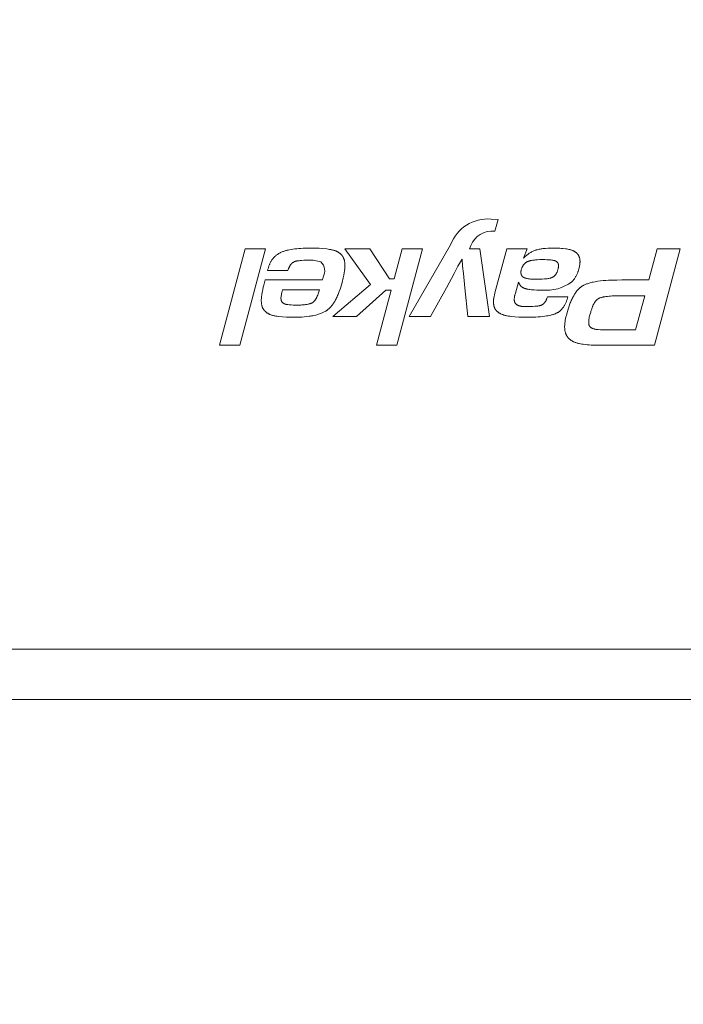
# Model space of a CAD drawing. Units: inches. Extents: x -1198 to -69, y -512 to 437.
# Tile 34 of 50: x -629.007 to -627.245, y 180.515 to 183.132. Entities that reach past the tile are written whole.
import ezdxf

# ---------------------------------------------------------------- set-up
doc = ezdxf.new("R2010")
doc.units = ezdxf.units.IN
doc.header["$MEASUREMENT"] = 0
for name, color, linetype, lineweight in [('0_Pen_No__7', 7, 'Continuous', 18), ('A-ANNO-DIMS', 2, 'Continuous', 18), ('A-EQPM', 60, 'Continuous', 18)]:
    doc.layers.add(name, color=color, linetype=linetype, lineweight=lineweight)
doc.styles.get("Standard").update_dxf_attribs({"font": 'arial.ttf'})
doc.dimstyles.get("Standard").update_dxf_attribs({"dimtxt": 6, "dimasz": 6, "dimexe": 0.18, "dimexo": 0.0625, "dimgap": 0.09, "dimtad": 0, "dimtih": 1, "dimtoh": 1, "dimdec": 0, "dimzin": 0, "dimdsep": 46, "dimlunit": 4, "dimtxsty": 'Standard', "dimblk": 'OBLIQUE', "dimcen": 0.09, "dimadec": 0, "dimazin": 0, "dimtfac": 1, "dimtdec": 0, "dimtofl": 0, "dimtmove": 0, "dimatfit": 3, "dimfxl": 1, "dimtolj": 1, "dimtzin": 0, "dimarcsym": 0})

# ---------------------------------------------------------------- blocks, each defined once
blk = doc.blocks.new('new block')
at = {"layer": '0_Pen_No__7'}
for p, q in [((-358.997, 99.109), (485.681, 99.109)), ((485.681, 95.73), (-358.997, 95.73)), ((-281.076, 68.7), (-279.346, 75.2)), ((-279.346, 75.2), (-275.605, 75.2)), ((-263.696, 68.7), (-261.965, 75.2)), ((-261.965, 75.2), (-260.589, 75.2)), ((-260.589, 75.2), (-261.574, 71.478)), ((-253.094, 68.7), (-251.364, 75.2)), ((-249.986, 75.2), (-251.716, 68.7)), ((-251.364, 75.2), (-249.986, 75.2)), ((-278.066, 74.168), (-278.675, 71.867)), ((-276.153, 74.168), (-278.066, 74.168)), ((-267.552, 68.7), (-268.209, 73.251)), ((-268.209, 73.251), (-266.747, 73.251)), ((-266.747, 73.251), (-266.552, 71.321)), ((-262.799, 73.251), (-265.577, 68.417)), ((-265.297, 71.321), (-264.224, 73.251)), ((-264.224, 73.251), (-262.799, 73.251)), ((-261.221, 71.478), (-259.224, 73.251)), ((-257.639, 73.251), (-260.186, 71.107)), ((-259.224, 73.251), (-257.639, 73.251)), ((-278.675, 71.867), (-276.921, 71.867)), ((-272.109, 71.935), (-273.497, 71.935)), ((-254.202, 71.634), (-254.141, 72.033)), ((-270.171, 70.951), (-269.953, 71.692)), ((-268.575, 71.673), (-269.367, 68.7)), ((-266.552, 71.321), (-266.443, 70.356)), ((-265.821, 70.356), (-265.297, 71.321)), ((-261.574, 71.478), (-261.221, 71.478)), ((-256.736, 71.458), (-254.251, 71.458)), ((-254.251, 71.458), (-254.202, 71.634)), ((-252.985, 71.146), (-253.081, 70.776)), ((-278.956, 70.795), (-279.517, 68.7)), ((-277.141, 70.795), (-278.956, 70.795)), ((-276.786, 70.805), (-277.141, 70.795)), ((-261.783, 70.717), (-262.318, 68.7)), ((-261.453, 70.717), (-261.783, 70.717)), ((-260.138, 68.7), (-261.453, 70.717)), ((-260.186, 71.107), (-258.444, 68.7)), ((-256.931, 70.776), (-256.98, 70.601)), ((-253.081, 70.776), (-256.931, 70.776)), ((-266.443, 70.356), (-266.393, 69.87)), ((-266.393, 69.87), (-266.37, 69.393)), ((-266.37, 69.393), (-266.076, 69.87)), ((-266.076, 69.87), (-265.821, 70.356)), ((-254.605, 70.152), (-253.239, 70.152)), ((-253.264, 70.065), (-253.277, 70.016)), ((-253.239, 70.152), (-253.264, 70.065)), ((-270.744, 68.7), (-270.512, 69.324)), ((-279.517, 68.7), (-281.076, 68.7)), ((-269.367, 68.7), (-270.744, 68.7)), ((-266.857, 68.7), (-267.552, 68.7)), ((-262.318, 68.7), (-263.696, 68.7)), ((-258.444, 68.7), (-260.138, 68.7)), ((-251.716, 68.7), (-253.094, 68.7)), ((-268.794, 66.703), (-268.575, 67.501)), ((-268.575, 67.501), (-268.307, 67.492)), ((-268.318, 66.683), (-268.794, 66.703))]:
    blk.add_line(p, q, dxfattribs=at)
for points in [[(-275.605, 75.2), (-275.335, 75.196), (-275.064, 75.185), (-274.929, 75.176), (-274.794, 75.164), (-274.659, 75.149), (-274.524, 75.132), (-274.432, 75.118), (-274.34, 75.102), (-274.249, 75.084), (-274.204, 75.074), (-274.159, 75.062), (-274.115, 75.05), (-274.071, 75.036), (-274.027, 75.022), (-273.983, 75.006), (-273.94, 74.989), (-273.898, 74.97), (-273.877, 74.96), (-273.856, 74.95), (-273.836, 74.939), (-273.815, 74.928), (-273.785, 74.911), (-273.755, 74.893), (-273.725, 74.874), (-273.696, 74.854), (-273.668, 74.833), (-273.64, 74.811), (-273.613, 74.789), (-273.586, 74.765), (-273.561, 74.741), (-273.537, 74.716), (-273.525, 74.703), (-273.513, 74.69), (-273.502, 74.677), (-273.49, 74.664), (-273.48, 74.65), (-273.469, 74.637), (-273.459, 74.623), (-273.449, 74.609), (-273.439, 74.594), (-273.43, 74.58), (-273.421, 74.565), (-273.412, 74.55), (-273.403, 74.534), (-273.394, 74.517), (-273.385, 74.5), (-273.377, 74.483), (-273.37, 74.466), (-273.362, 74.449), (-273.355, 74.431), (-273.349, 74.414), (-273.342, 74.396), (-273.336, 74.378), (-273.331, 74.36), (-273.326, 74.342), (-273.316, 74.305), (-273.307, 74.268), (-273.3, 74.23), (-273.294, 74.192), (-273.289, 74.154), (-273.285, 74.116), (-273.282, 74.077), (-273.279, 74.039), (-273.278, 74), (-273.277, 73.962), (-273.278, 73.905), (-273.28, 73.848), (-273.283, 73.792), (-273.288, 73.736), (-273.294, 73.68), (-273.302, 73.624), (-273.31, 73.569), (-273.32, 73.513), (-273.342, 73.403), (-273.367, 73.294), (-273.395, 73.185), (-273.425, 73.077)], [(-275.032, 72.969), (-274.96, 73.227), (-274.938, 73.314), (-274.929, 73.357), (-274.92, 73.401), (-274.913, 73.445), (-274.907, 73.489), (-274.902, 73.534), (-274.9, 73.556), (-274.899, 73.579), (-274.898, 73.602), (-274.898, 73.624), (-274.898, 73.647), (-274.898, 73.67), (-274.899, 73.687), (-274.9, 73.704), (-274.901, 73.722), (-274.903, 73.739), (-274.905, 73.756), (-274.908, 73.773), (-274.911, 73.789), (-274.915, 73.806), (-274.919, 73.822), (-274.923, 73.838), (-274.929, 73.854), (-274.935, 73.869), (-274.941, 73.884), (-274.949, 73.899), (-274.957, 73.913), (-274.966, 73.926), (-274.975, 73.938), (-274.984, 73.95), (-274.995, 73.961), (-275.006, 73.972), (-275.017, 73.982), (-275.029, 73.992), (-275.041, 74.002), (-275.054, 74.011), (-275.067, 74.02), (-275.081, 74.028), (-275.094, 74.036), (-275.108, 74.043), (-275.123, 74.05), (-275.137, 74.057), (-275.152, 74.064), (-275.166, 74.07), (-275.189, 74.078), (-275.212, 74.086), (-275.235, 74.094), (-275.258, 74.1), (-275.281, 74.106), (-275.305, 74.112), (-275.328, 74.116), (-275.352, 74.121), (-275.399, 74.128), (-275.446, 74.134), (-275.541, 74.143), (-275.694, 74.154), (-275.847, 74.162), (-276, 74.166), (-276.153, 74.168)], [(-273.497, 71.935), (-273.47, 72.026), (-273.441, 72.117), (-273.425, 72.162), (-273.409, 72.207), (-273.391, 72.252), (-273.373, 72.296), (-273.354, 72.339), (-273.334, 72.383), (-273.312, 72.425), (-273.29, 72.468), (-273.267, 72.509), (-273.243, 72.55), (-273.217, 72.59), (-273.191, 72.63), (-273.167, 72.662), (-273.143, 72.694), (-273.118, 72.726), (-273.092, 72.756), (-273.066, 72.786), (-273.038, 72.815), (-273.009, 72.842), (-272.995, 72.856), (-272.98, 72.869), (-272.951, 72.894), (-272.921, 72.917), (-272.891, 72.94), (-272.86, 72.961), (-272.829, 72.982), (-272.796, 73.001), (-272.764, 73.019), (-272.73, 73.037), (-272.71, 73.046), (-272.69, 73.056), (-272.65, 73.073), (-272.609, 73.09), (-272.567, 73.105), (-272.525, 73.119), (-272.483, 73.132), (-272.441, 73.145), (-272.398, 73.156), (-272.342, 73.17), (-272.287, 73.183), (-272.175, 73.206), (-272.063, 73.225), (-271.95, 73.242), (-271.796, 73.261), (-271.641, 73.276), (-271.485, 73.288), (-271.33, 73.297), (-271.019, 73.307), (-270.707, 73.31)], [(-270.707, 73.31), (-270.445, 73.307), (-270.183, 73.297), (-269.921, 73.28), (-269.659, 73.254), (-269.572, 73.243), (-269.484, 73.23), (-269.398, 73.215), (-269.354, 73.207), (-269.311, 73.198), (-269.268, 73.188), (-269.226, 73.176), (-269.184, 73.164), (-269.142, 73.151), (-269.1, 73.137), (-269.058, 73.121), (-269.017, 73.104), (-268.977, 73.085), (-268.949, 73.072), (-268.922, 73.058), (-268.895, 73.043), (-268.868, 73.027), (-268.842, 73.011), (-268.816, 72.994), (-268.791, 72.976), (-268.767, 72.957), (-268.743, 72.938), (-268.731, 72.928), (-268.72, 72.918), (-268.709, 72.907), (-268.698, 72.897), (-268.687, 72.886), (-268.677, 72.875), (-268.666, 72.864), (-268.656, 72.853), (-268.647, 72.841), (-268.637, 72.83), (-268.628, 72.818), (-268.619, 72.806), (-268.611, 72.793), (-268.602, 72.781), (-268.594, 72.768), (-268.586, 72.754), (-268.578, 72.741), (-268.571, 72.727), (-268.564, 72.713), (-268.557, 72.699), (-268.551, 72.685), (-268.545, 72.67), (-268.539, 72.655), (-268.534, 72.641), (-268.528, 72.626), (-268.523, 72.611), (-268.519, 72.596), (-268.514, 72.58), (-268.51, 72.565), (-268.506, 72.55), (-268.499, 72.518), (-268.494, 72.487), (-268.489, 72.455), (-268.484, 72.423), (-268.481, 72.391), (-268.479, 72.359), (-268.477, 72.327), (-268.477, 72.295), (-268.477, 72.255), (-268.478, 72.215), (-268.48, 72.175), (-268.483, 72.136), (-268.487, 72.097), (-268.492, 72.058), (-268.498, 72.019), (-268.504, 71.98), (-268.519, 71.902), (-268.536, 71.825), (-268.575, 71.673)], [(-258.26, 70.97), (-258.219, 71.12), (-258.175, 71.27), (-258.128, 71.418), (-258.077, 71.565), (-258.021, 71.711), (-257.992, 71.783), (-257.961, 71.854), (-257.929, 71.925), (-257.895, 71.995), (-257.86, 72.064), (-257.824, 72.133), (-257.794, 72.186), (-257.763, 72.239), (-257.732, 72.292), (-257.698, 72.343), (-257.664, 72.394), (-257.629, 72.444), (-257.592, 72.493), (-257.554, 72.54), (-257.519, 72.581), (-257.484, 72.62), (-257.448, 72.659), (-257.41, 72.696), (-257.371, 72.733), (-257.332, 72.767), (-257.311, 72.784), (-257.291, 72.801), (-257.27, 72.817), (-257.248, 72.833), (-257.226, 72.849), (-257.204, 72.864), (-257.181, 72.879), (-257.158, 72.894), (-257.111, 72.922), (-257.063, 72.948), (-257.014, 72.974), (-256.965, 72.997), (-256.914, 73.02), (-256.864, 73.041), (-256.803, 73.064), (-256.742, 73.086), (-256.681, 73.107), (-256.619, 73.126), (-256.557, 73.144), (-256.494, 73.16), (-256.368, 73.19), (-256.287, 73.207), (-256.205, 73.222), (-256.123, 73.236), (-256.04, 73.249), (-255.875, 73.27), (-255.709, 73.286), (-255.543, 73.297), (-255.376, 73.305), (-255.043, 73.31)], [(-255.043, 73.31), (-254.777, 73.306), (-254.512, 73.296), (-254.246, 73.278), (-253.98, 73.251), (-253.892, 73.241), (-253.804, 73.229), (-253.716, 73.214), (-253.673, 73.205), (-253.63, 73.196), (-253.587, 73.186), (-253.545, 73.174), (-253.503, 73.161), (-253.461, 73.147), (-253.42, 73.132), (-253.4, 73.124), (-253.38, 73.115), (-253.36, 73.106), (-253.34, 73.097), (-253.32, 73.087), (-253.301, 73.077), (-253.273, 73.062), (-253.246, 73.045), (-253.219, 73.028), (-253.192, 73.01), (-253.167, 72.991), (-253.142, 72.972), (-253.117, 72.951), (-253.093, 72.93), (-253.07, 72.908), (-253.059, 72.897), (-253.048, 72.886), (-253.037, 72.874), (-253.027, 72.862), (-253.016, 72.85), (-253.006, 72.838), (-252.997, 72.826), (-252.987, 72.813), (-252.978, 72.801), (-252.969, 72.788), (-252.96, 72.775), (-252.951, 72.762), (-252.943, 72.748), (-252.935, 72.735), (-252.927, 72.719), (-252.918, 72.704), (-252.91, 72.688), (-252.903, 72.672), (-252.896, 72.655), (-252.889, 72.639), (-252.882, 72.622), (-252.876, 72.606), (-252.871, 72.589), (-252.865, 72.572), (-252.86, 72.555), (-252.855, 72.537), (-252.851, 72.52), (-252.846, 72.503), (-252.839, 72.467), (-252.832, 72.432), (-252.827, 72.396), (-252.822, 72.36), (-252.819, 72.324), (-252.816, 72.288), (-252.814, 72.251), (-252.813, 72.215), (-252.813, 72.179), (-252.814, 72.122), (-252.816, 72.065), (-252.82, 72.009), (-252.825, 71.953), (-252.832, 71.897), (-252.839, 71.842), (-252.856, 71.731), (-252.883, 71.584), (-252.914, 71.437), (-252.948, 71.291), (-252.985, 71.146)], [(-276.921, 71.867), (-276.705, 71.869), (-276.488, 71.876), (-276.38, 71.882), (-276.272, 71.89), (-276.164, 71.901), (-276.056, 71.914), (-275.982, 71.925), (-275.908, 71.938), (-275.871, 71.946), (-275.834, 71.954), (-275.797, 71.963), (-275.761, 71.972), (-275.734, 71.98), (-275.708, 71.988), (-275.682, 71.997), (-275.656, 72.006), (-275.643, 72.011), (-275.63, 72.017), (-275.617, 72.022), (-275.605, 72.028), (-275.593, 72.034), (-275.58, 72.04), (-275.568, 72.047), (-275.556, 72.053), (-275.546, 72.06), (-275.535, 72.067), (-275.524, 72.074), (-275.514, 72.081), (-275.504, 72.089), (-275.494, 72.096), (-275.484, 72.104), (-275.474, 72.112), (-275.464, 72.121), (-275.455, 72.129), (-275.436, 72.146), (-275.418, 72.165), (-275.401, 72.183), (-275.381, 72.206), (-275.362, 72.229), (-275.343, 72.253), (-275.326, 72.277), (-275.309, 72.302), (-275.292, 72.327), (-275.277, 72.353), (-275.261, 72.379), (-275.242, 72.413), (-275.224, 72.449), (-275.206, 72.484), (-275.189, 72.52), (-275.173, 72.556), (-275.157, 72.593), (-275.128, 72.666), (-275.101, 72.741), (-275.077, 72.817), (-275.054, 72.893), (-275.032, 72.969)], [(-273.425, 73.077), (-273.465, 72.926), (-273.508, 72.776), (-273.555, 72.627), (-273.605, 72.479), (-273.66, 72.333), (-273.69, 72.261), (-273.72, 72.189), (-273.752, 72.118), (-273.786, 72.048), (-273.821, 71.978), (-273.857, 71.909), (-273.886, 71.856), (-273.916, 71.805), (-273.948, 71.753), (-273.98, 71.703), (-274.014, 71.653), (-274.049, 71.604), (-274.086, 71.557), (-274.124, 71.51), (-274.157, 71.471), (-274.192, 71.434), (-274.228, 71.397), (-274.264, 71.361), (-274.283, 71.344), (-274.303, 71.327), (-274.322, 71.311), (-274.342, 71.295), (-274.362, 71.279), (-274.382, 71.263), (-274.403, 71.249), (-274.424, 71.234), (-274.446, 71.219), (-274.469, 71.205), (-274.492, 71.191), (-274.515, 71.177), (-274.538, 71.164), (-274.562, 71.152), (-274.61, 71.128), (-274.659, 71.105), (-274.708, 71.084), (-274.759, 71.065), (-274.809, 71.046), (-274.873, 71.025), (-274.938, 71.004), (-275.002, 70.986), (-275.068, 70.969), (-275.133, 70.953), (-275.199, 70.938), (-275.331, 70.912), (-275.511, 70.882), (-275.692, 70.858), (-275.873, 70.84), (-276.056, 70.825), (-276.238, 70.816), (-276.421, 70.809), (-276.786, 70.805)], [(-270.854, 72.589), (-270.994, 72.587), (-271.133, 72.582), (-271.273, 72.573), (-271.413, 72.56), (-271.458, 72.554), (-271.503, 72.548), (-271.547, 72.541), (-271.569, 72.537), (-271.591, 72.532), (-271.612, 72.527), (-271.634, 72.521), (-271.655, 72.515), (-271.676, 72.508), (-271.686, 72.504), (-271.696, 72.5), (-271.706, 72.496), (-271.716, 72.491), (-271.726, 72.487), (-271.736, 72.482), (-271.746, 72.477), (-271.755, 72.472), (-271.77, 72.463), (-271.785, 72.454), (-271.8, 72.444), (-271.814, 72.434), (-271.828, 72.423), (-271.842, 72.411), (-271.855, 72.4), (-271.868, 72.388), (-271.881, 72.375), (-271.893, 72.362), (-271.905, 72.349), (-271.917, 72.336), (-271.928, 72.322), (-271.939, 72.308), (-271.949, 72.293), (-271.96, 72.279), (-271.973, 72.259), (-271.985, 72.239), (-271.997, 72.219), (-272.008, 72.198), (-272.019, 72.177), (-272.029, 72.156), (-272.039, 72.134), (-272.048, 72.113), (-272.057, 72.091), (-272.065, 72.069), (-272.081, 72.024), (-272.095, 71.98), (-272.109, 71.935)], [(-269.953, 71.692), (-269.937, 71.745), (-269.923, 71.797), (-269.91, 71.85), (-269.904, 71.876), (-269.899, 71.903), (-269.894, 71.93), (-269.89, 71.957), (-269.886, 71.984), (-269.883, 72.011), (-269.881, 72.038), (-269.879, 72.065), (-269.878, 72.093), (-269.878, 72.121), (-269.879, 72.136), (-269.879, 72.151), (-269.88, 72.166), (-269.881, 72.181), (-269.883, 72.196), (-269.885, 72.21), (-269.887, 72.225), (-269.89, 72.24), (-269.893, 72.254), (-269.897, 72.268), (-269.901, 72.282), (-269.906, 72.296), (-269.911, 72.309), (-269.917, 72.323), (-269.924, 72.335), (-269.931, 72.348), (-269.938, 72.359), (-269.946, 72.37), (-269.955, 72.381), (-269.964, 72.392), (-269.973, 72.402), (-269.983, 72.412), (-269.993, 72.421), (-270.004, 72.43), (-270.015, 72.439), (-270.026, 72.448), (-270.038, 72.456), (-270.05, 72.464), (-270.062, 72.471), (-270.074, 72.478), (-270.086, 72.485), (-270.098, 72.492), (-270.109, 72.498), (-270.12, 72.503), (-270.142, 72.513), (-270.164, 72.522), (-270.186, 72.531), (-270.209, 72.539), (-270.232, 72.546), (-270.255, 72.552), (-270.278, 72.558), (-270.301, 72.563), (-270.324, 72.568), (-270.348, 72.572), (-270.371, 72.576), (-270.395, 72.579), (-270.419, 72.581), (-270.467, 72.586), (-270.515, 72.588), (-270.564, 72.59), (-270.854, 72.589)], [(-255.226, 72.492), (-255.392, 72.49), (-255.475, 72.488), (-255.557, 72.484), (-255.64, 72.478), (-255.722, 72.47), (-255.804, 72.46), (-255.886, 72.448), (-255.944, 72.437), (-256.003, 72.424), (-256.032, 72.417), (-256.061, 72.41), (-256.089, 72.401), (-256.118, 72.392), (-256.14, 72.385), (-256.162, 72.377), (-256.184, 72.369), (-256.205, 72.36), (-256.215, 72.355), (-256.226, 72.35), (-256.236, 72.345), (-256.246, 72.339), (-256.256, 72.334), (-256.266, 72.328), (-256.276, 72.322), (-256.286, 72.315), (-256.294, 72.309), (-256.303, 72.303), (-256.312, 72.296), (-256.32, 72.29), (-256.328, 72.283), (-256.336, 72.275), (-256.344, 72.268), (-256.352, 72.261), (-256.36, 72.253), (-256.367, 72.245), (-256.382, 72.229), (-256.396, 72.213), (-256.41, 72.196), (-256.427, 72.175), (-256.443, 72.153), (-256.458, 72.13), (-256.473, 72.107), (-256.487, 72.084), (-256.501, 72.061), (-256.527, 72.013), (-256.544, 71.98), (-256.56, 71.947), (-256.576, 71.913), (-256.591, 71.879), (-256.619, 71.811), (-256.646, 71.741), (-256.67, 71.671), (-256.694, 71.6), (-256.736, 71.458)], [(-254.141, 72.033), (-254.141, 72.048), (-254.142, 72.063), (-254.143, 72.079), (-254.144, 72.094), (-254.146, 72.11), (-254.148, 72.125), (-254.151, 72.14), (-254.154, 72.155), (-254.157, 72.17), (-254.162, 72.185), (-254.166, 72.2), (-254.172, 72.214), (-254.178, 72.228), (-254.184, 72.242), (-254.191, 72.255), (-254.199, 72.268), (-254.207, 72.279), (-254.216, 72.29), (-254.224, 72.3), (-254.234, 72.31), (-254.244, 72.32), (-254.254, 72.329), (-254.264, 72.338), (-254.275, 72.347), (-254.287, 72.355), (-254.298, 72.363), (-254.31, 72.37), (-254.322, 72.377), (-254.335, 72.384), (-254.347, 72.391), (-254.36, 72.397), (-254.373, 72.403), (-254.382, 72.407), (-254.392, 72.411), (-254.411, 72.418), (-254.431, 72.425), (-254.451, 72.431), (-254.471, 72.436), (-254.491, 72.441), (-254.511, 72.445), (-254.531, 72.449), (-254.552, 72.453), (-254.572, 72.456), (-254.613, 72.461), (-254.696, 72.469), (-254.828, 72.479), (-254.961, 72.487), (-255.094, 72.491), (-255.226, 72.492)], [(-271.755, 71.478), (-271.579, 71.477), (-271.403, 71.472), (-271.227, 71.463), (-271.051, 71.451), (-270.936, 71.44), (-270.879, 71.433), (-270.822, 71.425), (-270.765, 71.415), (-270.737, 71.409), (-270.709, 71.403), (-270.681, 71.396), (-270.653, 71.388), (-270.625, 71.38), (-270.598, 71.371), (-270.579, 71.364), (-270.561, 71.357), (-270.542, 71.349), (-270.524, 71.342), (-270.506, 71.333), (-270.488, 71.325), (-270.47, 71.316), (-270.453, 71.306), (-270.436, 71.296), (-270.419, 71.285), (-270.403, 71.275), (-270.387, 71.263), (-270.371, 71.251), (-270.356, 71.239), (-270.341, 71.226), (-270.327, 71.212), (-270.313, 71.199), (-270.301, 71.185), (-270.288, 71.17), (-270.276, 71.155), (-270.265, 71.14), (-270.254, 71.124), (-270.243, 71.108), (-270.233, 71.091), (-270.223, 71.075), (-270.214, 71.058), (-270.206, 71.04), (-270.198, 71.023), (-270.19, 71.005), (-270.183, 70.987), (-270.177, 70.97), (-270.171, 70.951)], [(-270.512, 69.324), (-270.556, 69.278), (-270.601, 69.234), (-270.646, 69.191), (-270.693, 69.149), (-270.741, 69.108), (-270.791, 69.069), (-270.841, 69.031), (-270.893, 68.995), (-270.941, 68.964), (-270.991, 68.934), (-271.041, 68.905), (-271.092, 68.878), (-271.144, 68.853), (-271.197, 68.83), (-271.251, 68.808), (-271.305, 68.788), (-271.335, 68.778), (-271.366, 68.768), (-271.429, 68.75), (-271.492, 68.734), (-271.555, 68.72), (-271.619, 68.708), (-271.684, 68.697), (-271.748, 68.688), (-271.813, 68.679), (-271.894, 68.67), (-271.975, 68.663), (-272.138, 68.652), (-272.324, 68.645), (-272.511, 68.642), (-272.735, 68.645), (-272.847, 68.649), (-272.958, 68.655), (-273.054, 68.662), (-273.149, 68.671), (-273.339, 68.693), (-273.411, 68.703), (-273.484, 68.715), (-273.556, 68.729), (-273.591, 68.736), (-273.627, 68.745), (-273.662, 68.754), (-273.697, 68.764), (-273.732, 68.775), (-273.766, 68.787), (-273.8, 68.8), (-273.834, 68.814), (-273.85, 68.822), (-273.867, 68.83), (-273.883, 68.838), (-273.9, 68.846), (-273.923, 68.859), (-273.946, 68.873), (-273.969, 68.887), (-273.991, 68.902), (-274.013, 68.918), (-274.034, 68.934), (-274.055, 68.951), (-274.075, 68.969), (-274.095, 68.987), (-274.104, 68.996), (-274.114, 69.006), (-274.123, 69.015), (-274.132, 69.025), (-274.141, 69.035), (-274.149, 69.045), (-274.158, 69.056), (-274.166, 69.066), (-274.174, 69.077), (-274.182, 69.087), (-274.189, 69.098), (-274.196, 69.109), (-274.203, 69.12), (-274.21, 69.132), (-274.217, 69.144), (-274.224, 69.156), (-274.23, 69.168), (-274.236, 69.18), (-274.242, 69.193), (-274.247, 69.205), (-274.253, 69.218), (-274.258, 69.231), (-274.262, 69.244), (-274.267, 69.257), (-274.271, 69.27), (-274.275, 69.283), (-274.283, 69.31), (-274.29, 69.337), (-274.295, 69.364), (-274.3, 69.392), (-274.304, 69.419), (-274.308, 69.447), (-274.31, 69.475), (-274.312, 69.503), (-274.313, 69.531), (-274.314, 69.558), (-274.313, 69.587), (-274.312, 69.615), (-274.311, 69.644), (-274.309, 69.672), (-274.306, 69.7), (-274.303, 69.728), (-274.295, 69.784), (-274.284, 69.848), (-274.272, 69.91), (-274.257, 69.973), (-274.241, 70.036), (-274.216, 70.124), (-274.188, 70.213), (-274.173, 70.256), (-274.157, 70.3), (-274.14, 70.343), (-274.123, 70.385), (-274.104, 70.428), (-274.084, 70.469), (-274.064, 70.511), (-274.042, 70.551), (-274.02, 70.592), (-273.996, 70.631), (-273.971, 70.67), (-273.946, 70.708), (-273.924, 70.737), (-273.902, 70.766), (-273.88, 70.795), (-273.856, 70.823), (-273.832, 70.85), (-273.808, 70.877), (-273.783, 70.903), (-273.757, 70.929)], [(-271.438, 70.747), (-271.611, 70.745), (-271.771, 70.739), (-271.917, 70.729), (-271.984, 70.723), (-272.048, 70.716), (-272.108, 70.708), (-272.164, 70.699), (-272.217, 70.688), (-272.267, 70.677), (-272.291, 70.671), (-272.314, 70.665), (-272.336, 70.658), (-272.358, 70.651), (-272.379, 70.644), (-272.399, 70.636), (-272.419, 70.629), (-272.438, 70.62), (-272.457, 70.612), (-272.474, 70.603), (-272.491, 70.593), (-272.508, 70.584), (-272.524, 70.574), (-272.54, 70.563), (-272.555, 70.552), (-272.57, 70.541), (-272.584, 70.529), (-272.598, 70.516), (-272.611, 70.503), (-272.624, 70.49), (-272.637, 70.476), (-272.649, 70.461), (-272.661, 70.446), (-272.672, 70.431), (-272.683, 70.414), (-272.694, 70.397), (-272.704, 70.38), (-272.715, 70.362), (-272.724, 70.343), (-272.734, 70.324), (-272.743, 70.305), (-272.752, 70.285), (-272.761, 70.265), (-272.769, 70.244), (-272.785, 70.202), (-272.8, 70.158), (-272.814, 70.114), (-272.824, 70.078), (-272.834, 70.042), (-272.842, 70.006), (-272.85, 69.97), (-272.853, 69.952), (-272.856, 69.934), (-272.859, 69.917), (-272.861, 69.899), (-272.862, 69.882), (-272.863, 69.865), (-272.864, 69.848), (-272.864, 69.832), (-272.864, 69.817), (-272.863, 69.802), (-272.862, 69.788), (-272.86, 69.773), (-272.858, 69.76), (-272.855, 69.746), (-272.852, 69.733), (-272.849, 69.72), (-272.845, 69.707), (-272.841, 69.694), (-272.836, 69.682), (-272.831, 69.67), (-272.825, 69.659), (-272.819, 69.648), (-272.813, 69.637), (-272.806, 69.626), (-272.799, 69.616), (-272.791, 69.606), (-272.783, 69.597), (-272.775, 69.587), (-272.766, 69.578), (-272.756, 69.57), (-272.746, 69.562), (-272.736, 69.554), (-272.725, 69.546), (-272.713, 69.538), (-272.701, 69.531), (-272.688, 69.525), (-272.675, 69.518), (-272.661, 69.512), (-272.647, 69.506), (-272.632, 69.5), (-272.617, 69.495), (-272.601, 69.49), (-272.584, 69.485), (-272.567, 69.481), (-272.549, 69.476), (-272.53, 69.472), (-272.491, 69.465), (-272.448, 69.458), (-272.403, 69.452), (-272.355, 69.446), (-272.304, 69.441), (-272.191, 69.433), (-272.067, 69.427), (-271.929, 69.423), (-271.78, 69.422)], [(-270.33, 70.309), (-270.33, 70.324), (-270.331, 70.338), (-270.332, 70.353), (-270.333, 70.367), (-270.335, 70.381), (-270.337, 70.394), (-270.34, 70.408), (-270.343, 70.421), (-270.347, 70.433), (-270.351, 70.446), (-270.356, 70.458), (-270.361, 70.469), (-270.367, 70.481), (-270.373, 70.492), (-270.379, 70.503), (-270.386, 70.514), (-270.394, 70.524), (-270.402, 70.534), (-270.411, 70.544), (-270.42, 70.554), (-270.429, 70.563), (-270.439, 70.572), (-270.45, 70.581), (-270.461, 70.59), (-270.473, 70.598), (-270.486, 70.606), (-270.499, 70.614), (-270.512, 70.621), (-270.526, 70.629), (-270.541, 70.636), (-270.556, 70.643), (-270.572, 70.649), (-270.589, 70.656), (-270.606, 70.662), (-270.624, 70.668), (-270.642, 70.673), (-270.661, 70.679), (-270.681, 70.684), (-270.723, 70.694), (-270.767, 70.703), (-270.813, 70.711), (-270.863, 70.718), (-270.915, 70.724), (-270.97, 70.73), (-271.028, 70.735), (-271.152, 70.742), (-271.289, 70.746), (-271.438, 70.747)], [(-253.277, 70.016), (-253.288, 69.973), (-253.301, 69.929), (-253.314, 69.886), (-253.328, 69.844), (-253.344, 69.801), (-253.36, 69.759), (-253.378, 69.717), (-253.396, 69.676), (-253.416, 69.635), (-253.436, 69.595), (-253.458, 69.555), (-253.481, 69.516), (-253.505, 69.478), (-253.53, 69.441), (-253.556, 69.404), (-253.583, 69.368), (-253.611, 69.335), (-253.639, 69.303), (-253.668, 69.271), (-253.698, 69.241), (-253.729, 69.211), (-253.76, 69.182), (-253.793, 69.154), (-253.826, 69.127), (-253.86, 69.101), (-253.895, 69.076), (-253.93, 69.052), (-253.966, 69.028), (-254.003, 69.006), (-254.04, 68.985), (-254.078, 68.964), (-254.116, 68.945), (-254.164, 68.922), (-254.212, 68.9), (-254.261, 68.88), (-254.311, 68.862), (-254.361, 68.844), (-254.412, 68.828), (-254.463, 68.813), (-254.514, 68.799), (-254.566, 68.786), (-254.618, 68.774), (-254.722, 68.753), (-254.827, 68.734), (-254.932, 68.718), (-255.069, 68.699), (-255.205, 68.684), (-255.341, 68.671), (-255.478, 68.661), (-255.637, 68.653), (-255.796, 68.647), (-256.115, 68.642), (-256.417, 68.645), (-256.568, 68.65), (-256.718, 68.658), (-256.971, 68.677), (-257.224, 68.703), (-257.317, 68.714), (-257.41, 68.728), (-257.502, 68.743), (-257.548, 68.752), (-257.593, 68.762), (-257.639, 68.773), (-257.684, 68.785), (-257.728, 68.798), (-257.772, 68.813), (-257.816, 68.829), (-257.837, 68.837), (-257.859, 68.846), (-257.88, 68.856), (-257.901, 68.866), (-257.922, 68.876), (-257.943, 68.887), (-257.972, 68.902), (-258.001, 68.919), (-258.029, 68.937), (-258.057, 68.955), (-258.084, 68.975), (-258.11, 68.995), (-258.136, 69.016), (-258.161, 69.038), (-258.173, 69.049), (-258.185, 69.061), (-258.197, 69.073), (-258.209, 69.084), (-258.22, 69.096), (-258.231, 69.109), (-258.242, 69.121), (-258.252, 69.134), (-258.263, 69.147), (-258.273, 69.16), (-258.282, 69.173), (-258.292, 69.186), (-258.301, 69.2), (-258.31, 69.214), (-258.318, 69.228), (-258.327, 69.242), (-258.335, 69.257), (-258.343, 69.272), (-258.351, 69.288), (-258.358, 69.304), (-258.365, 69.32), (-258.372, 69.336), (-258.378, 69.352), (-258.384, 69.369), (-258.39, 69.385), (-258.396, 69.402), (-258.406, 69.435), (-258.415, 69.469), (-258.423, 69.503), (-258.43, 69.542), (-258.437, 69.582), (-258.443, 69.621), (-258.447, 69.661), (-258.45, 69.701), (-258.453, 69.741), (-258.454, 69.781), (-258.455, 69.82), (-258.454, 69.882), (-258.451, 69.943), (-258.446, 70.004), (-258.441, 70.065), (-258.433, 70.126), (-258.425, 70.187), (-258.406, 70.309), (-258.375, 70.475), (-258.34, 70.641), (-258.26, 70.97)], [(-271.78, 69.422), (-271.607, 69.424), (-271.446, 69.431), (-271.3, 69.441), (-271.232, 69.448), (-271.168, 69.456), (-271.107, 69.465), (-271.049, 69.474), (-270.995, 69.485), (-270.969, 69.491), (-270.944, 69.497), (-270.92, 69.504), (-270.897, 69.511), (-270.874, 69.518), (-270.852, 69.525), (-270.83, 69.533), (-270.809, 69.541), (-270.789, 69.55), (-270.769, 69.558), (-270.749, 69.568), (-270.73, 69.578), (-270.711, 69.589), (-270.693, 69.6), (-270.676, 69.611), (-270.659, 69.623), (-270.642, 69.635), (-270.626, 69.648), (-270.61, 69.661), (-270.595, 69.675), (-270.581, 69.689), (-270.566, 69.704), (-270.552, 69.719), (-270.539, 69.734), (-270.526, 69.75), (-270.513, 69.767), (-270.5, 69.784), (-270.488, 69.802), (-270.476, 69.82), (-270.464, 69.838), (-270.453, 69.857), (-270.442, 69.877), (-270.432, 69.898), (-270.421, 69.919), (-270.411, 69.941), (-270.402, 69.963), (-270.393, 69.986), (-270.384, 70.009), (-270.376, 70.033), (-270.368, 70.056), (-270.354, 70.103), (-270.346, 70.132), (-270.339, 70.159), (-270.336, 70.173), (-270.334, 70.186), (-270.331, 70.198), (-270.33, 70.211), (-270.328, 70.227), (-270.328, 70.242), (-270.328, 70.256), (-270.328, 70.269), (-270.33, 70.305)], [(-255.982, 69.46), (-255.827, 69.462), (-255.672, 69.467), (-255.518, 69.476), (-255.44, 69.483), (-255.362, 69.492), (-255.315, 69.498), (-255.267, 69.505), (-255.22, 69.513), (-255.196, 69.518), (-255.173, 69.523), (-255.149, 69.529), (-255.126, 69.535), (-255.104, 69.542), (-255.081, 69.55), (-255.059, 69.558), (-255.037, 69.567), (-255.026, 69.572), (-255.015, 69.577), (-255.005, 69.582), (-254.994, 69.587), (-254.978, 69.596), (-254.962, 69.605), (-254.947, 69.615), (-254.931, 69.625), (-254.916, 69.636), (-254.902, 69.647), (-254.888, 69.658), (-254.874, 69.67), (-254.866, 69.677), (-254.859, 69.684), (-254.845, 69.698), (-254.831, 69.713), (-254.818, 69.728), (-254.805, 69.744), (-254.792, 69.759), (-254.78, 69.776), (-254.769, 69.792), (-254.755, 69.813), (-254.742, 69.834), (-254.729, 69.855), (-254.717, 69.877), (-254.705, 69.899), (-254.694, 69.921), (-254.683, 69.943), (-254.673, 69.966), (-254.663, 69.989), (-254.654, 70.012), (-254.636, 70.058), (-254.62, 70.105), (-254.605, 70.152)]]:
    blk.add_lwpolyline(points, dxfattribs=at)
for centre, radius, start, end in [((-272.026, 68.543), 2.947, 84.73509, 125.96945), ((-256.236, 70.185), 0.852, 150.77527, 225.45817), ((-256.103, 71.739), 2.282, 251.32192, 273.04529), ((-268.413, 69.092), 1.604, 273.78097, 345.86999), ((-268.106, 69.382), 2.707, 265.51181, 339.11597)]:
    blk.add_arc(centre, radius, start, end, dxfattribs=at)
blk = doc.blocks.new('_Oblique')
at = {"color": 0, "linetype": 'ByBlock', "lineweight": -2}
blk.add_line((-0.5, -0.5), (0.5, 0.5), dxfattribs=at)
blk = doc.blocks.new('*D56')
at = {"layer": 'A-ANNO-DIMS', "color": 0, "lineweight": -2, "ltscale": 10, "transparency": 16777216}
for p, q in [((-618.3394, 257.2277), (-603.8219, 257.2277)), ((-604.0019, 257.2277), (-604.0019, 212.422)), ((-604.0019, 161.2277), (-604.0019, 206.0333)), ((-618.3394, 161.2277), (-603.8219, 161.2277))]:
    blk.add_line(p, q, dxfattribs=at)
at = {"layer": 'DEFPOINTS', "color": 0, "ltscale": 10, "transparency": 16777216}
for p in [(-618.4019, 257.2277), (-604.0019, 257.2277), (-618.4019, 161.2277)]:
    blk.add_point(p, dxfattribs=at)
at = {"layer": 'A-ANNO-DIMS', "color": 0, "lineweight": -2, "ltscale": 10, "transparency": 16777216, "xscale": 6, "yscale": 6, "zscale": 6}
for p, rotation in [((-604.0019, 257.2277), 90), ((-604.0019, 161.2277), 270)]:
    blk.add_blockref('_Oblique', p, dxfattribs=dict(at, rotation=rotation))
at = {"layer": 'A-ANNO-DIMS', "color": 0, "ltscale": 10, "transparency": 16777216, "insert": (-604.0019, 209.2277), "char_height": 6, "attachment_point": 5}
blk.add_mtext('\\A1;COUNTER 96 TYP.', dxfattribs=at)

msp = doc.modelspace()

# ---------------------------------------------------------------- block references
at = {"layer": 'A-EQPM', "xscale": 0.0393700787401575, "yscale": 0.0393700787401575, "zscale": 0.0393700787401575, "rotation": 180}
msp.add_blockref('new block', (-638.3186, 185.2277), dxfattribs=at)

# ---------------------------------------------------------------- dimensions: what is measured, and where the dimension line sits
at = {"layer": 'A-ANNO-DIMS', "ltscale": 10}
dim = msp.add_linear_dim(base=(-604.0019, 257.2277), p1=(-618.4019, 161.2277), p2=(-618.4019, 257.2277), angle=90, text='COUNTER <> TYP.', dimstyle='Standard', override={"dimdec": 0, "dimlfac": 1, "dimrnd": 0, "dimzin": 0, "dimdsep": 46, "dimlunit": 2}, dxfattribs=at)
dim.commit()
dim.dimension.update_dxf_attribs({"geometry": '*D56', "text_midpoint": (-604.0019, 209.2277)})

doc.saveas('drawing.dxf')
